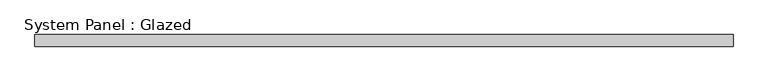
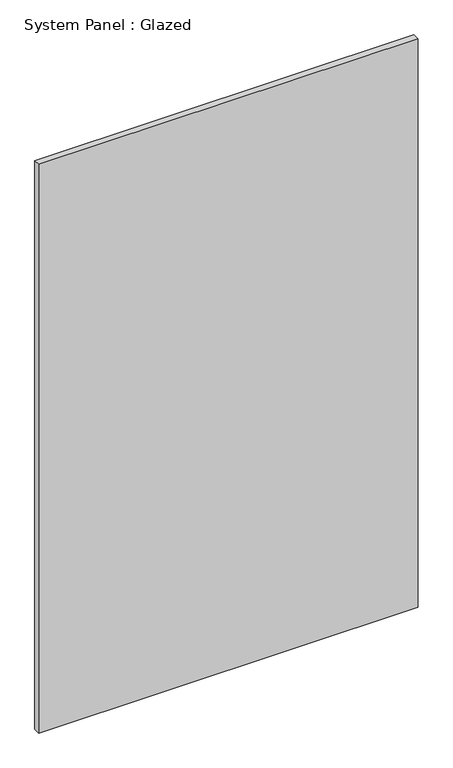
"""IFC4 building model written with IfcOpenShell, lengths in millimetres: plate geometry, System Panel : Glazed."""

from ifc_helpers import new_model, si_unit, origin, origin_with_axes, place, context, project, spatial, polyline, outline, extrude, source, transform, mapped, element, save


def system_panel_glazed_97fa76a5(model_context):
    return source(origin(), model_context, "Body", "SweptSolid", [
        extrude(outline(polyline([(739.3657433, -44.45), (-739.3657433, -44.45), (-739.3657433, -19.05), (739.3657433, -19.05), (739.3657433, -44.45)])), origin_with_axes(), (0.0, 0.0, 1.0), 2343.15),
    ])


if __name__ == "__main__":
    model = new_model("IFC4")
    model_context = context("Model", 3, world=origin())
    ifc_project = project(units=[si_unit("LENGTHUNIT", "METRE", prefix="MILLI")], contexts=[model_context])
    site = spatial("IfcSite", under=ifc_project)
    building = spatial("IfcBuilding", under=site)
    placement = place(None, origin())
    system_panel_glazed_shape = system_panel_glazed_97fa76a5(model_context)
    element("IfcPlate", 1, ObjectType="System Panel : Glazed", at=placement, inside=building, context=model_context, shape_type="MappedRepresentation", body=[
        mapped(system_panel_glazed_shape, transform((0.0, 0.0, 0.0), x_axis=(1.0, 0.0, 0.0), y_axis=(0.0, 1.0, 0.0), z_axis=(0.0, 0.0, 1.0))),
    ])
    save(model, "model.ifc")

# Revit data of these elements
# Type "System Panel : Glazed"
#   Construction Type Id = "GSP4R"
#   Analytic Construction = "1/8 in Pilkington single glazing"
#   Visual Light Transmittance = 0.9
#   Solar Heat Gain Coefficient = 0.86
#   Heat Transfer Coefficient (U) = 1.18115 BTU/(h·ft²·°F)
# Element 1 (IfcPlate, "System Panel : Glazed")
#   Materials on its faces: "Glass"
# Materials
#   "Glass": class "Glass", colour RGB 0 128 192, transparency 0.75, Description = "Soda Lime Glass", Cost = 0
